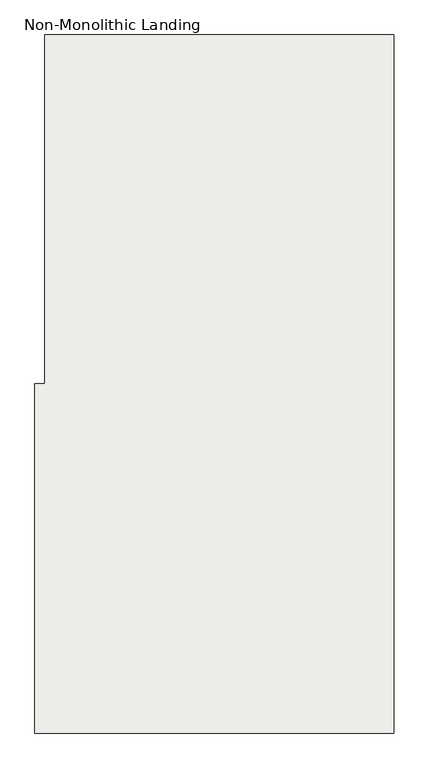
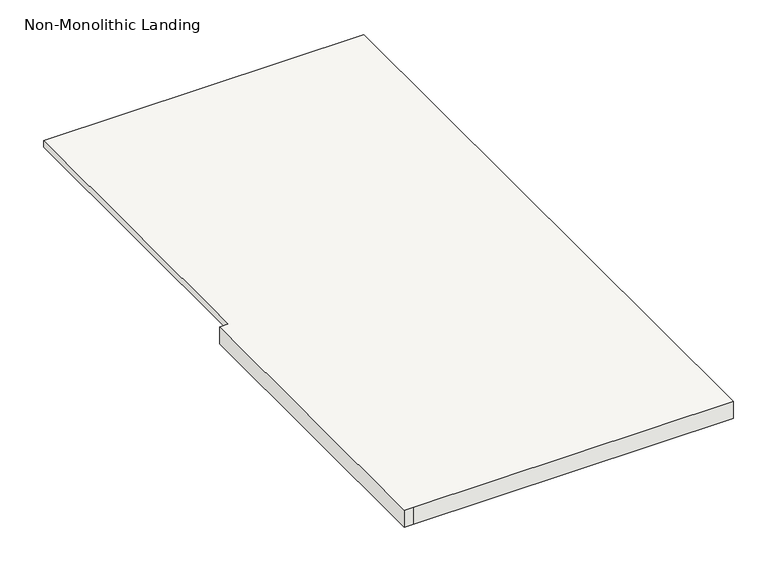
"""IFC4 building model written with IfcOpenShell, lengths in millimetres: slab geometry, Non-Monolithic Landing."""

from ifc_helpers import new_model, si_unit, origin, place, context, project, spatial, faceted_brep, source, transform, mapped, element, save


def non_monolithic_landing_66cdc52a(model_context):
    return source(origin(), model_context, "Body", "Brep", [
        faceted_brep([(-6294.6389568, 4109.9342758, 1524.0), (-6294.6389568, 4109.9342758, 1504.95), (-6294.6389568, 3195.5342758, 1504.95), (-6294.6389568, 3195.5342758, 1524.0), (-6269.2389568, 4109.9342758, 1479.55), (-6269.2389568, 3195.5342758, 1479.55), (-6320.0389568, 3195.5342758, 1524.0), (-6320.0389568, 2281.1342758, 1524.0), (-6294.6389568, 2281.1342758, 1524.0), (-5380.2389568, 2281.1342758, 1524.0), (-5380.2389568, 4109.9342758, 1524.0), (-6269.2389568, 3195.5342758, 1473.2), (-6269.2389568, 4109.9342758, 1473.2), (-5380.2389568, 4109.9342758, 1473.2), (-5380.2389568, 2281.1342758, 1473.2), (-6294.6389568, 2281.1342758, 1473.2), (-6320.0389568, 2281.1342758, 1473.2), (-6320.0389568, 3195.5342758, 1473.2)], [[[0, 1, 2, 3]], [[1, 4, 5, 2]], [[6, 7, 8, 9, 10, 0, 3]], [[11, 12, 13, 14, 15, 16, 17]], [[12, 11, 5, 4]], [[11, 17, 6, 3, 2, 5]], [[7, 6, 17, 16]], [[8, 7, 16, 15]], [[9, 8, 15, 14]], [[10, 9, 14, 13]], [[0, 10, 13, 12, 4, 1]]]),
    ])


if __name__ == "__main__":
    model = new_model("IFC4")
    model_context = context("Model", 3, world=origin())
    ifc_project = project(units=[si_unit("LENGTHUNIT", "METRE", prefix="MILLI")], contexts=[model_context])
    site = spatial("IfcSite", under=ifc_project)
    building = spatial("IfcBuilding", under=site)
    placement = place(None, origin())
    non_monolithic_landing_shape = non_monolithic_landing_66cdc52a(model_context)
    element("IfcSlab", 1, ObjectType="Non-Monolithic Landing", at=placement, inside=building, context=model_context, shape_type="MappedRepresentation", body=[
        mapped(non_monolithic_landing_shape, transform((0.0, 0.0, 0.0), x_axis=(1.0, 0.0, 0.0), y_axis=(0.0, 1.0, 0.0), z_axis=(0.0, 0.0, 1.0))),
    ])
    save(model, "model.ifc")
